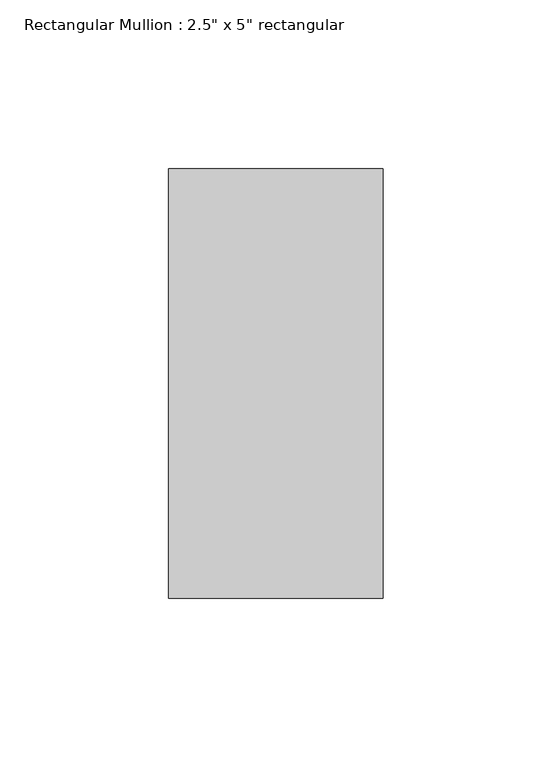
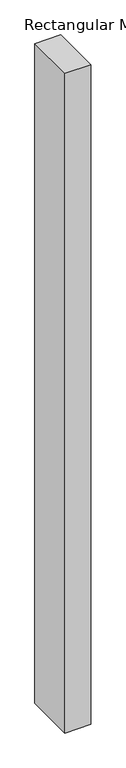
"""IFC4 building model written with IfcOpenShell, lengths in millimetres: member geometry."""

from ifc_helpers import new_model, si_unit, frame, origin, place, context, project, spatial, polyline, outline, extrude, source, transform, mapped, element, save


def member_b8ac15de(model_context):
    return source(origin(), model_context, "Body", "SweptSolid", [
        extrude(outline(polyline([(31.75, 63.5), (31.75, -63.5), (-31.75, -63.5), (-31.75, 63.5), (31.75, 63.5)])), frame((0.0, 0.0, -1707.486558), z_axis=(0.0, 0.0, 1.0), x_axis=(1.0, 0.0, 0.0)), (0.0, 0.0, 1.0), 1707.486558),
    ])


if __name__ == "__main__":
    model = new_model("IFC4")
    model_context = context("Model", 3, world=origin())
    ifc_project = project(units=[si_unit("LENGTHUNIT", "METRE", prefix="MILLI")], contexts=[model_context])
    site = spatial("IfcSite", under=ifc_project)
    building = spatial("IfcBuilding", under=site)
    placement = place(None, origin())
    member_shape = member_b8ac15de(model_context)
    element("IfcMember", 1, ObjectType="Rectangular Mullion : 2.5\" x 5\" rectangular", at=placement, inside=building, context=model_context, shape_type="MappedRepresentation", body=[
        mapped(member_shape, transform((0.0, 0.0, 0.0), x_axis=(1.0, 0.0, 0.0), y_axis=(0.0, 1.0, 0.0), z_axis=(0.0, 0.0, 1.0))),
    ])
    save(model, "model.ifc")

# Revit data of these elements
# Type "Rectangular Mullion : 2.5\" x 5\" rectangular"
#   built-in parameter 1007304 = 0.416667 (stored number, unit not read)
#   built-in parameter 1007301 = 0.104167 (stored number, unit not read)
#   built-in parameter 1007300 = 0.104167 (stored number, unit not read)
# Element 1 (IfcMember, "Rectangular Mullion : 2.5\" x 5\" rectangular")
#   Materials on its faces: "Aluminum"
# Materials
#   "Aluminum": class "Metal", colour RGB 247 247 247, transparency 0, Description = "Aluminum 6061", Cost = 0
